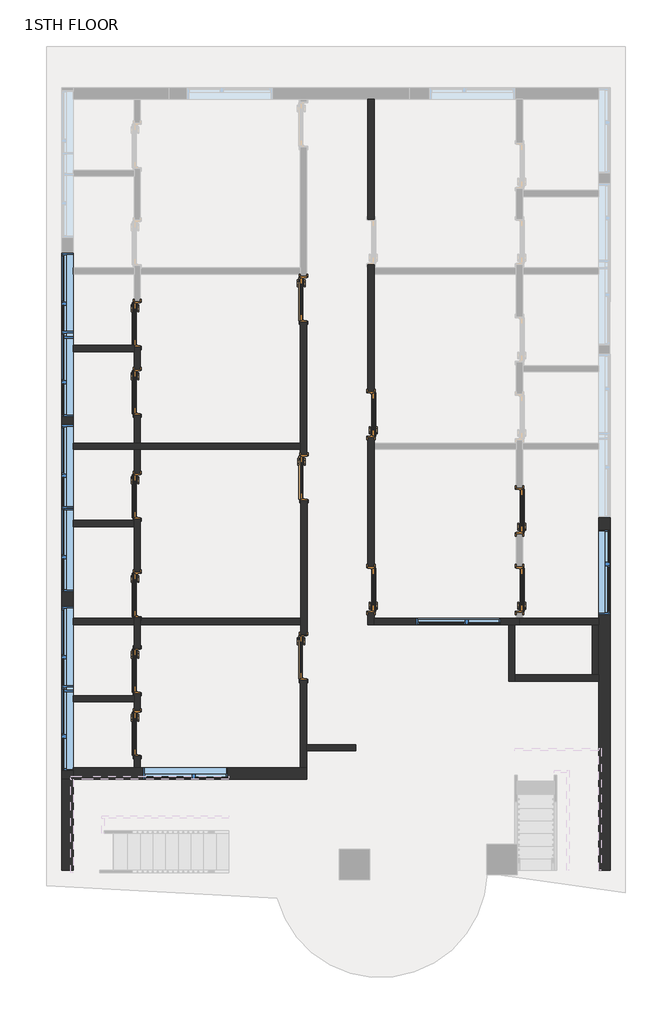
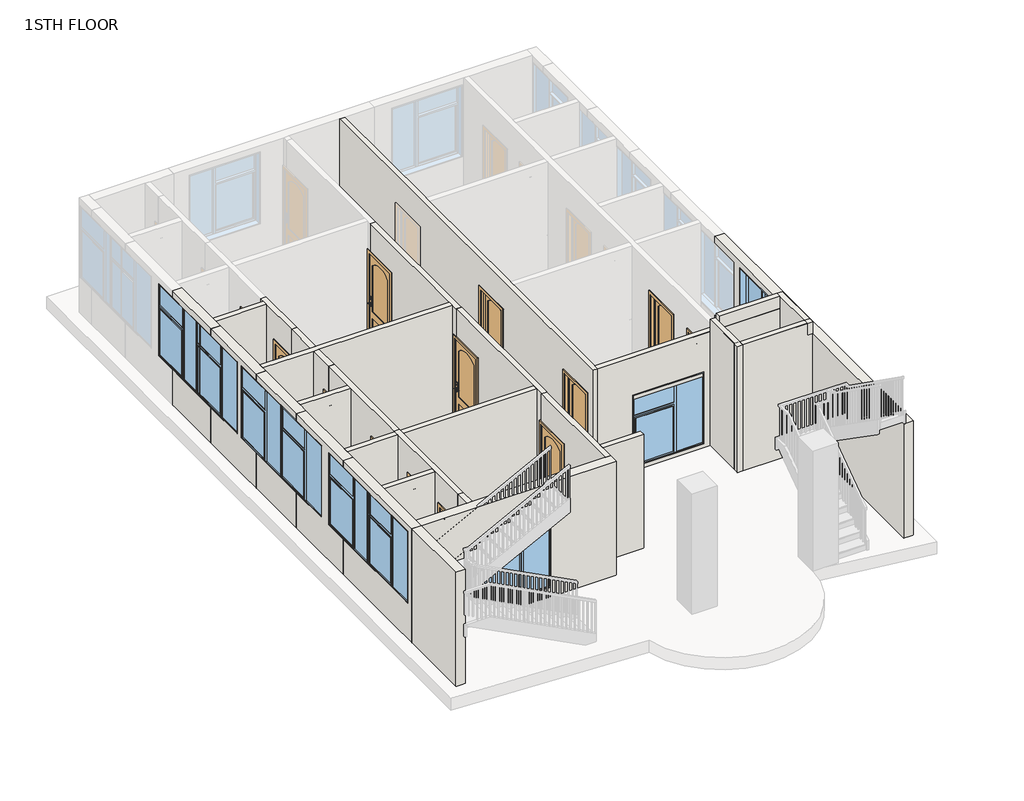
# One storey, part 1 of 4: 32 walls, 13 doors, 9 windows.
"""IFC4 building model written with IfcOpenShell, lengths in millimetres."""

from ifc_helpers import new_model, si_unit, frame, origin, place, context, project, spatial, polyline, outline, extrude, faceted_brep, transform, mapped, element, save
from components import door_346b4a94, m_window_casement_double_sidelight_1702_x_1829mm_c8b42c7f, m_window_casement_double_sidelight_1702_x_1829mm_92594323

model = new_model("IFC4")

# Units and contexts
model_context = context("Model", 3, world=origin())
ifc_project = project(units=[si_unit("LENGTHUNIT", "METRE", prefix="MILLI")], contexts=[model_context])

# Site, building, storey
site = spatial("IfcSite", under=ifc_project)
building = spatial("IfcBuilding", under=site)
storey = spatial("IfcBuildingStorey", under=building, Name="1STH FLOOR", Elevation=3200.4)

# Doors
placement = place(None, origin())
door_shape = door_346b4a94(model_context)
element("IfcDoor", 1, ObjectType="2'10\"X7'", at=placement, inside=storey, context=model_context, shape_type="MappedRepresentation", body=[
    mapped(door_shape, transform((2698.7641134, -459.3600272, 3200.4), x_axis=(0.0, -1.0, 0.0), y_axis=(1.0, 0.0, 0.0), z_axis=(0.0, 0.0, 1.0))),
])
element("IfcDoor", 2, ObjectType="2'10\"X7'", at=placement, inside=storey, context=model_context, shape_type="MappedRepresentation", body=[
    mapped(door_shape, transform((2698.7641134, -2034.1600272, 3200.4), x_axis=(0.0, -1.0, 0.0), y_axis=(1.0, 0.0, 0.0), z_axis=(0.0, 0.0, 1.0))),
])
element("IfcDoor", 3, ObjectType="2'10\"X7'", at=placement, inside=storey, context=model_context, shape_type="MappedRepresentation", body=[
    mapped(door_shape, transform((-273.0358866, -2034.1600272, 3200.4), x_axis=(0.0, -1.0, 0.0), y_axis=(1.0, 0.0, 0.0), z_axis=(0.0, 0.0, 1.0))),
])
element("IfcDoor", 4, ObjectType="2'10\"X7'", at=placement, inside=storey, context=model_context, shape_type="MappedRepresentation", body=[
    mapped(door_shape, transform((-273.0358866, 1471.0399728, 3200.4), x_axis=(0.0, -1.0, 0.0), y_axis=(1.0, 0.0, 0.0), z_axis=(0.0, 0.0, 1.0))),
])
element("IfcDoor", 5, ObjectType="2'10\"X7'", at=placement, inside=storey, context=model_context, shape_type="MappedRepresentation", body=[
    mapped(door_shape, transform((-4952.9858866, -3659.7600272, 3200.4), x_axis=(0.0, 1.0, 0.0), y_axis=(-1.0, 0.0, 0.0), z_axis=(0.0, 0.0, 1.0))),
])
element("IfcDoor", 6, ObjectType="2'10\"X7'", at=placement, inside=storey, context=model_context, shape_type="MappedRepresentation", body=[
    mapped(door_shape, transform((-4952.9858866, -2142.5151651, 3200.4), x_axis=(0.0, 1.0, 0.0), y_axis=(-1.0, 0.0, 0.0), z_axis=(0.0, 0.0, 1.0))),
])
element("IfcDoor", 7, ObjectType="2'10\"X7'", at=placement, inside=storey, context=model_context, shape_type="MappedRepresentation", body=[
    mapped(door_shape, transform((-4952.9858866, -167.9704957, 3200.4), x_axis=(0.0, 1.0, 0.0), y_axis=(-1.0, 0.0, 0.0), z_axis=(0.0, 0.0, 1.0))),
])
element("IfcDoor", 8, ObjectType="2'10\"X7'", at=placement, inside=storey, context=model_context, shape_type="MappedRepresentation", body=[
    mapped(door_shape, transform((-4952.9858866, 3273.6174518, 3200.4), x_axis=(0.0, 1.0, 0.0), y_axis=(-1.0, 0.0, 0.0), z_axis=(0.0, 0.0, 1.0))),
])
element("IfcDoor", 9, ObjectType="2'10\"X7'", at=placement, inside=storey, context=model_context, shape_type="MappedRepresentation", body=[
    mapped(door_shape, transform((-1625.1621817, 3775.8008884, 3200.4), x_axis=(0.0, 1.0, 0.0), y_axis=(-1.0, 0.0, 0.0), z_axis=(0.0, 0.0, 1.0))),
])
element("IfcDoor", 10, ObjectType="2'10\"X7'", at=placement, inside=storey, context=model_context, shape_type="MappedRepresentation", body=[
    mapped(door_shape, transform((-1629.1419858, -3390.4626067, 3200.4), x_axis=(0.0, 1.0, 0.0), y_axis=(-1.0, 0.0, 0.0), z_axis=(0.0, 0.0, 1.0))),
])
element("IfcDoor", 11, ObjectType="2'10\"X7'", at=placement, inside=storey, context=model_context, shape_type="MappedRepresentation", body=[
    mapped(door_shape, transform((-1620.1577262, 202.9637706, 3200.4), x_axis=(0.0, 1.0, 0.0), y_axis=(-1.0, 0.0, 0.0), z_axis=(0.0, 0.0, 1.0))),
])
element("IfcDoor", 12, ObjectType="2'10\"X7'", at=placement, inside=storey, context=model_context, shape_type="MappedRepresentation", body=[
    mapped(door_shape, transform((-4952.9858866, -4917.0600272, 3200.4), x_axis=(0.0, 1.0, 0.0), y_axis=(-1.0, 0.0, 0.0), z_axis=(0.0, 0.0, 1.0))),
])
element("IfcDoor", 13, ObjectType="2'10\"X7'", at=placement, inside=storey, context=model_context, shape_type="MappedRepresentation", body=[
    mapped(door_shape, transform((-4952.9858866, 1913.3521609, 3200.4), x_axis=(0.0, 1.0, 0.0), y_axis=(-1.0, 0.0, 0.0), z_axis=(0.0, 0.0, 1.0))),
])

# Walls
element("IfcWall", 14, ObjectType="Generic - 4.5\"", at=placement, inside=storey, context=model_context, shape_type="Brep", body=[
    faceted_brep([(-6232.5508078, 2728.3399728, 3200.4), (-5013.3108866, 2728.3399728, 3200.4), (-5013.3108866, 2728.3399728, 6096.0), (-6232.5508078, 2728.3399728, 6096.0), (-6232.5508078, 2855.3399728, 3200.4), (-6232.5508078, 2855.3399728, 6096.0), (-5013.3108866, 2855.3399728, 6096.0), (-5013.3108866, 2855.3399728, 3200.4), (-5013.3108866, 2816.8174518, 3200.4)], [[[0, 1, 2, 3]], [[4, 5, 6, 7]], [[1, 0, 4, 7, 8]], [[0, 3, 5, 4]], [[2, 1, 8, 7, 6]], [[3, 2, 6, 5]]]),
])
element("IfcWall", 15, ObjectType="Generic - 4.5\"", at=placement, inside=storey, context=model_context, shape_type="Brep", body=[
    faceted_brep([(-5013.3108866, 2968.8174518, 6096.0), (-5013.3108866, 2968.8174518, 5359.0), (-5013.3108866, 2816.8174518, 5359.0), (-5013.3108866, 2816.8174518, 3200.4), (-5013.3108866, 2728.3399728, 3200.4), (-5013.3108866, 2370.1521609, 3200.4), (-5013.3108866, 2370.1521609, 5359.0), (-5013.3108866, 1684.7521609, 5359.0), (-5013.3108866, 1684.7521609, 6096.0), (-5013.3108866, 2728.3399728, 6096.0), (-5013.3108866, 2855.3399728, 6096.0), (-4886.3108866, 2968.8174518, 5359.0), (-4886.3108866, 2968.8174518, 6096.0), (-4886.3108866, 1684.7521609, 6096.0), (-4886.3108866, 1684.7521609, 5359.0), (-4886.3108866, 2370.1521609, 5359.0), (-4886.3108866, 2370.1521609, 3200.4), (-4886.3108866, 2816.8174518, 3200.4), (-4886.3108866, 2816.8174518, 5359.0)], [[[0, 1, 2, 3, 4, 5, 6, 7, 8, 9, 10]], [[11, 12, 13, 14, 15, 16, 17, 18]], [[3, 17, 16, 5, 4]], [[13, 8, 7, 14]], [[1, 0, 12, 11]], [[18, 2, 1, 11]], [[2, 18, 17, 3]], [[15, 6, 5, 16]], [[6, 15, 14, 7]], [[0, 10, 9, 8, 13, 12]]]),
])
element("IfcWall", 16, ObjectType="Generic - 4.5\"", at=placement, inside=storey, context=model_context, shape_type="Brep", body=[
    faceted_brep([(-6232.5508078, 772.5399728, 3200.4), (-5013.3108866, 772.5399728, 3200.4), (-4886.3108866, 772.5399728, 3200.4), (-1685.9108866, 772.5399728, 3200.4), (-1685.9108866, 772.5399728, 6096.0), (-4886.3108866, 772.5399728, 6096.0), (-5013.3108866, 772.5399728, 6096.0), (-6232.5508078, 772.5399728, 6096.0), (-6232.5508078, 899.5399728, 3200.4), (-6232.5508078, 899.5399728, 6096.0), (-5013.3108866, 899.5399728, 6096.0), (-4886.3108866, 899.5399728, 6096.0), (-1685.9108866, 899.5399728, 6096.0), (-1685.9108866, 899.5399728, 3200.4), (-4886.3108866, 899.5399728, 3200.4), (-5013.3108866, 899.5399728, 3200.4)], [[[0, 1, 2, 3, 4, 5, 6, 7]], [[8, 9, 10, 11, 12, 13, 14, 15]], [[3, 2, 1, 0, 8, 15, 14, 13]], [[4, 3, 13, 12]], [[0, 7, 9, 8]], [[7, 6, 5, 4, 12, 11, 10, 9]]]),
])
element("IfcWall", 17, ObjectType="Generic - 4.5\"", at=placement, inside=storey, context=model_context, shape_type="SweptSolid", body=[
    extrude(outline(polyline([(136.8295043, 5359.0), (136.8295043, 6096.0), (772.5399728, 6096.0), (772.5399728, 3200.4), (288.8295043, 3200.4), (288.8295043, 5359.0), (136.8295043, 5359.0)])), frame((-5013.3108866, 0.0, 0.0), z_axis=(1.0, 0.0, 0.0), x_axis=(0.0, 1.0, 0.0)), (0.0, 0.0, 1.0), 127.0),
    extrude(outline(polyline([(1684.7521609, 6096.0), (1684.7521609, 5359.0), (1456.5521609, 5359.0), (1456.5521609, 3200.4), (899.5399728, 3200.4), (899.5399728, 6096.0), (1684.7521609, 6096.0)])), frame((-5013.3108866, 0.0, 0.0), z_axis=(1.0, 0.0, 0.0), x_axis=(0.0, 1.0, 0.0)), (0.0, 0.0, 1.0), 127.0),
])
element("IfcWall", 18, ObjectType="Generic - 4.5\"", at=placement, inside=storey, context=model_context, shape_type="SweptSolid", body=[
    extrude(outline(polyline([(-5013.3108866, -776.8600272), (-6232.5508078, -776.8600272), (-6232.5508078, -649.8600272), (-5013.3108866, -649.8600272), (-5013.3108866, -776.8600272)])), frame((0.0, 0.0, 3200.4), z_axis=(0.0, 0.0, 1.0), x_axis=(1.0, 0.0, 0.0)), (0.0, 0.0, 1.0), 2895.6),
])
element("IfcWall", 19, ObjectType="Generic - 4.5\"", at=placement, inside=storey, context=model_context, shape_type="Brep", body=[
    faceted_brep([(-5013.3108866, -2574.3151651, 5359.0), (-5013.3108866, -2574.3151651, 6096.0), (-5013.3108866, -776.8600272, 6096.0), (-5013.3108866, -649.8600272, 6096.0), (-5013.3108866, 136.8295043, 6096.0), (-5013.3108866, 136.8295043, 5359.0), (-5013.3108866, -624.7704957, 5359.0), (-5013.3108866, -624.7704957, 3200.4), (-5013.3108866, -649.8600272, 3200.4), (-5013.3108866, -776.8600272, 3200.4), (-5013.3108866, -1685.7151651, 3200.4), (-5013.3108866, -1685.7151651, 5359.0), (-4886.3108866, -2574.3151651, 6096.0), (-4886.3108866, -2574.3151651, 5359.0), (-4886.3108866, -1685.7151651, 5359.0), (-4886.3108866, -1685.7151651, 3200.4), (-4886.3108866, -624.7704957, 3200.4), (-4886.3108866, -624.7704957, 5359.0), (-4886.3108866, 136.8295043, 5359.0), (-4886.3108866, 136.8295043, 6096.0)], [[[0, 1, 2, 3, 4, 5, 6, 7, 8, 9, 10, 11]], [[12, 13, 14, 15, 16, 17, 18, 19]], [[15, 10, 9, 8, 7, 16]], [[1, 0, 13, 12]], [[4, 19, 18, 5]], [[14, 11, 10, 15]], [[11, 14, 13, 0]], [[17, 6, 5, 18]], [[6, 17, 16, 7]], [[4, 3, 2, 1, 12, 19]]]),
])
element("IfcWall", 20, ObjectType="Generic - 4.5\"", at=placement, inside=storey, context=model_context, shape_type="SweptSolid", body=[
    extrude(outline(polyline([(-5013.3108866, -2732.6600272), (-6232.5508078, -2732.6600272), (-6232.5508078, -2605.6600272), (-5013.3108866, -2605.6600272), (-5013.3108866, -2732.6600272)])), frame((0.0, 0.0, 3200.4), z_axis=(0.0, 0.0, 1.0), x_axis=(1.0, 0.0, 0.0)), (0.0, 0.0, 1.0), 2895.6),
])
element("IfcWall", 21, ObjectType="Generic - 4.5\"", at=placement, inside=storey, context=model_context, shape_type="Brep", body=[
    faceted_brep([(-5013.3108866, -3202.9600272, 3200.4), (-5013.3108866, -3202.9600272, 5359.0), (-5013.3108866, -4116.5600272, 5359.0), (-5013.3108866, -4116.5600272, 3200.4), (-5013.3108866, -4155.0600272, 3200.4), (-5013.3108866, -4282.0600272, 3200.4), (-5013.3108866, -4460.2600272, 3200.4), (-5013.3108866, -4460.2600272, 5359.0), (-5013.3108866, -5221.8600272, 5359.0), (-5013.3108866, -5221.8600272, 6096.0), (-5013.3108866, -4282.0600272, 6096.0), (-5013.3108866, -4155.0600272, 6096.0), (-5013.3108866, -2732.6600272, 6096.0), (-5013.3108866, -2605.6600272, 6096.0), (-5013.3108866, -2574.3151651, 6096.0), (-5013.3108866, -2574.3151651, 5359.0), (-5013.3108866, -2599.3151651, 5359.0), (-5013.3108866, -2599.3151651, 3200.4), (-5013.3108866, -2605.6600272, 3200.4), (-5013.3108866, -2732.6600272, 3200.4), (-4886.3108866, -3202.9600272, 5359.0), (-4886.3108866, -3202.9600272, 3200.4), (-4886.3108866, -2732.6600272, 3200.4), (-4886.3108866, -2605.6600272, 3200.4), (-4886.3108866, -2599.3151651, 3200.4), (-4886.3108866, -2599.3151651, 5359.0), (-4886.3108866, -2574.3151651, 5359.0), (-4886.3108866, -2574.3151651, 6096.0), (-4886.3108866, -2605.6600272, 6096.0), (-4886.3108866, -2732.6600272, 6096.0), (-4886.3108866, -5221.8600272, 6096.0), (-4886.3108866, -5221.8600272, 5359.0), (-4886.3108866, -4460.2600272, 5359.0), (-4886.3108866, -4460.2600272, 3200.4), (-4886.3108866, -4116.5600272, 3200.4), (-4886.3108866, -4116.5600272, 5359.0)], [[[0, 1, 2, 3, 4, 5, 6, 7, 8, 9, 10, 11, 12, 13, 14, 15, 16, 17, 18, 19]], [[20, 21, 22, 23, 24, 25, 26, 27, 28, 29, 30, 31, 32, 33, 34, 35]], [[21, 0, 19, 18, 17, 24, 23, 22]], [[3, 34, 33, 6, 5, 4]], [[30, 9, 8, 31]], [[15, 14, 27, 26]], [[20, 1, 0, 21]], [[1, 20, 35, 2]], [[2, 35, 34, 3]], [[25, 16, 15, 26]], [[16, 25, 24, 17]], [[32, 7, 6, 33]], [[7, 32, 31, 8]], [[14, 13, 12, 11, 10, 9, 30, 29, 28, 27]]]),
])
element("IfcWall", 22, ObjectType="Generic - 4.5\"", at=placement, inside=storey, context=model_context, shape_type="SweptSolid", body=[
    extrude(outline(polyline([(-5013.3108866, -4282.0600272), (-6232.5324766, -4282.0600272), (-6232.5342541, -4155.0600272), (-5013.3108866, -4155.0600272), (-5013.3108866, -4282.0600272)])), frame((0.0, 0.0, 3200.4), z_axis=(0.0, 0.0, 1.0), x_axis=(1.0, 0.0, 0.0)), (0.0, 0.0, 1.0), 2895.6),
])
element("IfcWall", 23, ObjectType="Generic - 4.5\"", at=placement, inside=storey, context=model_context, shape_type="SweptSolid", body=[
    extrude(outline(polyline([(-1685.9108866, -2732.6600272), (-4886.3108866, -2732.6600272), (-4886.3108866, -2605.6600272), (-1685.9108866, -2605.6600272), (-1685.9108866, -2732.6600272)])), frame((0.0, 0.0, 3200.4), z_axis=(0.0, 0.0, 1.0), x_axis=(1.0, 0.0, 0.0)), (0.0, 0.0, 1.0), 2895.6),
])
element("IfcWall", 24, ObjectType="Generic - 4.5\"", at=placement, inside=storey, context=model_context, shape_type="Brep", body=[
    faceted_brep([(-1685.4871817, 4182.2008884, 6096.0), (-1685.4871817, 4182.2008884, 5359.0), (-1685.4871817, 3319.0008884, 5359.0), (-1685.4871817, 3319.0008884, 3200.4), (-1685.4871817, 659.7637706, 3200.4), (-1685.4871817, 659.7637706, 5359.0), (-1685.4871817, 609.3637706, 5359.0), (-1685.4871817, 609.3637706, 6096.0), (-1558.4871817, 4182.2008884, 5359.0), (-1558.4871817, 4182.2008884, 6096.0), (-1558.4871817, 609.3637706, 6096.0), (-1558.4871817, 609.3637706, 5359.0), (-1558.4871817, 659.7637706, 5359.0), (-1558.4871817, 659.7637706, 3200.4), (-1558.4871817, 3319.0008884, 3200.4), (-1558.4871817, 3319.0008884, 5359.0), (-1680.4827262, 609.3637706, 6096.0), (-1680.4827262, 609.3637706, 5359.0), (-1558.9108866, 4182.2008884, 6096.0), (-1558.9108866, 4182.2008884, 5359.0)], [[[0, 1, 2, 3, 4, 5, 6, 7]], [[8, 9, 10, 11, 12, 13, 14, 15]], [[3, 14, 13, 4]], [[10, 16, 7, 6, 17, 11]], [[1, 0, 18, 9, 8, 19]], [[15, 2, 1, 19, 8]], [[2, 15, 14, 3]], [[12, 5, 4, 13]], [[5, 12, 11, 17, 6]], [[0, 7, 16, 10, 9, 18]]]),
])
element("IfcWall", 25, ObjectType="Generic - 4.5\"", at=placement, inside=storey, context=model_context, shape_type="Brep", body=[
    faceted_brep([(-1680.4827262, -2933.2626067, 3200.4), (-1680.4827262, -2933.2626067, 6096.0), (-1680.4827262, 609.3637706, 6096.0), (-1680.4827262, 609.3637706, 5359.0), (-1680.4827262, -253.8362294, 5359.0), (-1680.4827262, -253.8362294, 3200.4), (-1553.4827262, -2933.2626067, 6096.0), (-1553.4827262, -2933.2626067, 3200.4), (-1553.4827262, -253.8362294, 3200.4), (-1553.4827262, -253.8362294, 5359.0), (-1553.4827262, 609.3637706, 5359.0), (-1553.4827262, 609.3637706, 6096.0), (-1562.4669858, -2933.2626067, 3200.4), (-1562.4669858, -2933.2626067, 6096.0), (-1558.4871817, 609.3637706, 6096.0), (-1558.4871817, 609.3637706, 5359.0)], [[[0, 1, 2, 3, 4, 5]], [[6, 7, 8, 9, 10, 11]], [[7, 12, 0, 5, 8]], [[1, 0, 12, 7, 6, 13]], [[2, 14, 11, 10, 15, 3]], [[9, 4, 3, 15, 10]], [[4, 9, 8, 5]], [[2, 1, 13, 6, 11, 14]]]),
])
element("IfcWall", 26, ObjectType="Generic - 4.5\"", at=placement, inside=storey, context=model_context, shape_type="Brep", body=[
    faceted_brep([(-1689.4669858, -2933.2626067, 6096.0), (-1689.4669858, -2933.2626067, 3200.4), (-1689.4669858, -2933.6626067, 3200.4), (-1689.4669858, -2933.6626067, 5359.0), (-1689.4669858, -3847.2626067, 5359.0), (-1689.4669858, -3847.2626067, 3200.4), (-1689.4669858, -5596.1082131, 3200.4), (-1689.4669858, -5596.1082131, 6096.0), (-1562.4669858, -2933.2626067, 3200.4), (-1562.4669858, -2933.2626067, 6096.0), (-1562.4669858, -5136.3822004, 6096.0), (-1562.4669858, -5263.3822004, 6096.0), (-1562.4669858, -5596.1082131, 6096.0), (-1562.4669858, -5596.1082131, 3200.4), (-1562.4669858, -5263.3822004, 3200.4), (-1562.4669858, -5136.3822004, 3200.4), (-1562.4669858, -3847.2626067, 3200.4), (-1562.4669858, -3847.2626067, 5359.0), (-1562.4669858, -2933.6626067, 5359.0), (-1562.4669858, -2933.6626067, 3200.4), (-1680.4827262, -2933.2626067, 3200.4), (-1680.4827262, -2933.2626067, 6096.0)], [[[0, 1, 2, 3, 4, 5, 6, 7]], [[8, 9, 10, 11, 12, 13, 14, 15, 16, 17, 18, 19]], [[1, 20, 8, 19, 2]], [[13, 6, 5, 16, 15, 14]], [[1, 0, 21, 9, 8, 20]], [[18, 3, 2, 19]], [[3, 18, 17, 4]], [[4, 17, 16, 5]], [[7, 6, 13, 12]], [[0, 7, 12, 11, 10, 9, 21]]]),
])
element("IfcWall", 27, ObjectType="Generic - 4.5\"", at=placement, inside=storey, context=model_context, shape_type="Brep", body=[
    faceted_brep([(-339.7108866, 7782.9399728, 6096.0), (-339.7108866, 7782.9399728, 3200.4), (-339.7108866, 5382.2399728, 3200.4), (-339.7108866, 5382.2399728, 5359.0), (-339.7108866, 4468.6399728, 5359.0), (-339.7108866, 4468.6399728, 3200.4), (-339.7108866, 1927.8399728, 3200.4), (-339.7108866, 1927.8399728, 5359.0), (-339.7108866, 1014.2399728, 5359.0), (-339.7108866, 1014.2399728, 3200.4), (-339.7108866, -1577.3600272, 3200.4), (-339.7108866, -1577.3600272, 5359.0), (-339.7108866, -2490.9600272, 5359.0), (-339.7108866, -2490.9600272, 3200.4), (-339.7108866, -2732.6600272, 3200.4), (-339.7108866, -2732.6600272, 6096.0), (-212.7108866, 7782.9399728, 3200.4), (-212.7108866, 7782.9399728, 6096.0), (-212.7108866, 4404.7399728, 6096.0), (-212.7108866, 4277.7399728, 6096.0), (-212.7108866, 899.5399728, 6096.0), (-212.7108866, 772.5399728, 6096.0), (-212.7108866, -2605.6600272, 6096.0), (-212.7108866, -2732.6600272, 6096.0), (-212.7108866, -2732.6600272, 3200.4), (-212.7108866, -2605.6600272, 3200.4), (-212.7108866, -2490.9600272, 3200.4), (-212.7108866, -2490.9600272, 5359.0), (-212.7108866, -1577.3600272, 5359.0), (-212.7108866, -1577.3600272, 3200.4), (-212.7108866, 772.5399728, 3200.4), (-212.7108866, 899.5399728, 3200.4), (-212.7108866, 1014.2399728, 3200.4), (-212.7108866, 1014.2399728, 5359.0), (-212.7108866, 1927.8399728, 5359.0), (-212.7108866, 1927.8399728, 3200.4), (-212.7108866, 4277.7399728, 3200.4), (-212.7108866, 4404.7399728, 3200.4), (-212.7108866, 4468.6399728, 3200.4), (-212.7108866, 4468.6399728, 5359.0), (-212.7108866, 5382.2399728, 5359.0), (-212.7108866, 5382.2399728, 3200.4)], [[[0, 1, 2, 3, 4, 5, 6, 7, 8, 9, 10, 11, 12, 13, 14, 15]], [[16, 17, 18, 19, 20, 21, 22, 23, 24, 25, 26, 27, 28, 29, 30, 31, 32, 33, 34, 35, 36, 37, 38, 39, 40, 41]], [[1, 16, 41, 2]], [[24, 14, 13, 26, 25]], [[29, 10, 9, 32, 31, 30]], [[35, 6, 5, 38, 37, 36]], [[1, 0, 17, 16]], [[15, 14, 24, 23]], [[12, 27, 26, 13]], [[27, 12, 11, 28]], [[28, 11, 10, 29]], [[8, 33, 32, 9]], [[33, 8, 7, 34]], [[34, 7, 6, 35]], [[4, 39, 38, 5]], [[39, 4, 3, 40]], [[40, 3, 2, 41]], [[0, 15, 23, 22, 21, 20, 19, 18, 17]]]),
])
element("IfcWall", 28, ObjectType="Generic - 4.5\"", at=placement, inside=storey, context=model_context, shape_type="Brep", body=[
    faceted_brep([(-212.7108866, -2732.6600272, 6096.0), (-212.7108866, -2732.6600272, 3200.4), (625.4891134, -2732.6600272, 3200.4), (625.4891134, -2732.6600272, 5014.5114654), (2327.2891134, -2732.6600272, 5014.5114654), (2327.2891134, -2732.6600272, 3200.4), (2479.6891134, -2732.6600272, 3200.4), (2606.6891134, -2732.6600272, 3200.4), (4281.7311655, -2732.6600272, 3200.4), (4281.7311655, -2732.6600272, 6096.0), (-212.7108866, -2605.6600272, 3200.4), (-212.7108866, -2605.6600272, 6096.0), (2632.0891134, -2605.6600272, 6096.0), (2759.0891134, -2605.6600272, 6096.0), (4281.7311655, -2605.6600272, 6096.0), (4281.7311655, -2605.6600272, 3200.4), (2759.0891134, -2605.6600272, 3200.4), (2632.0891134, -2605.6600272, 3200.4), (2327.2891134, -2605.6600272, 3200.4), (2327.2891134, -2605.6600272, 5014.5114654), (625.4891134, -2605.6600272, 5014.5114654), (625.4891134, -2605.6600272, 3200.4)], [[[0, 1, 2, 3, 4, 5, 6, 7, 8, 9]], [[10, 11, 12, 13, 14, 15, 16, 17, 18, 19, 20, 21]], [[1, 10, 21, 2]], [[15, 8, 7, 6, 5, 18, 17, 16]], [[1, 0, 11, 10]], [[9, 8, 15, 14]], [[0, 9, 14, 13, 12, 11]], [[20, 3, 2, 21]], [[4, 19, 18, 5]], [[3, 20, 19, 4]]]),
])
element("IfcWall", 29, ObjectType="Generic - 4.5\"", at=placement, inside=storey, context=model_context, shape_type="Brep", body=[
    faceted_brep([(-212.7108866, -2732.6600272, 3200.4), (2479.6891134, -2732.6600272, 3200.4), (2606.6891134, -2732.6600272, 3200.4), (2695.5891134, -2732.6600272, 3200.4), (2695.5891134, -2732.6600272, 6096.0), (-212.7108866, -2732.6600272, 6096.0), (625.4891134, -2732.6600272, 5126.3883506), (2327.2891134, -2732.6600272, 5126.3883506), (2327.2891134, -2732.6600272, 3297.5883506), (625.4891134, -2732.6600272, 3297.5883506), (-212.7108866, -2605.6600272, 3200.4), (-212.7108866, -2605.6600272, 6096.0), (2632.0891134, -2605.6600272, 6096.0), (2695.5891134, -2605.6600272, 6096.0), (2695.5891134, -2605.6600272, 3200.4), (2632.0891134, -2605.6600272, 3200.4), (625.4891134, -2605.6600272, 5126.3883506), (625.4891134, -2605.6600272, 3297.5883506), (2327.2891134, -2605.6600272, 3297.5883506), (2327.2891134, -2605.6600272, 5126.3883506)], [[[0, 1, 2, 3, 4, 5], [6, 7, 8, 9]], [[10, 11, 12, 13, 14, 15], [16, 17, 18, 19]], [[3, 2, 1, 0, 10, 15, 14]], [[4, 3, 14, 13]], [[5, 4, 13, 12, 11]], [[17, 16, 6, 9]], [[18, 17, 9, 8]], [[19, 18, 8, 7]], [[16, 19, 7, 6]], [[0, 5, 11, 10]]]),
])
element("IfcWall", 30, ObjectType="Generic - 5\"", at=placement, inside=storey, context=model_context, shape_type="SweptSolid", body=[
    extrude(outline(polyline([(-5593.5822004, 3200.4), (-5593.5822004, 6096.0), (-5221.8600272, 6096.0), (-5221.8600272, 5359.0), (-5373.8600272, 5359.0), (-5373.8600272, 3200.4), (-5593.5822004, 3200.4)])), frame((-5013.3108866, 0.0, 0.0), z_axis=(1.0, 0.0, 0.0), x_axis=(0.0, 1.0, 0.0)), (0.0, 0.0, 1.0), 127.0),
])
element("IfcWall", 31, ObjectType="Generic - 5\"", at=placement, inside=storey, context=model_context, shape_type="SweptSolid", body=[
    extrude(outline(polyline([(-1562.4669858, -5136.3822004), (-581.0108866, -5136.3822004), (-581.0108866, -5263.3822004), (-1562.4669858, -5263.3822004), (-1562.4669858, -5136.3822004)])), frame((0.0, 0.0, 3200.4), z_axis=(0.0, 0.0, 1.0), x_axis=(1.0, 0.0, 0.0)), (0.0, 0.0, 1.0), 2895.6),
])
element("IfcWall", 32, ObjectType="Generic - 5\"", at=placement, inside=storey, context=model_context, shape_type="Brep", body=[
    faceted_brep([(2479.6891134, -2732.6600272, 3200.4), (2479.6891134, -3866.3822004, 3200.4), (2479.6891134, -3866.3822004, 6400.8), (2479.6891134, -2732.6600272, 6400.8), (2606.6891134, -2732.6600272, 3200.4), (2606.6891134, -2732.6600272, 6400.8), (2606.6891134, -3739.3822004, 6400.8), (2606.6891134, -3866.3822004, 6400.8), (2606.6891134, -3866.3822004, 3200.4), (2606.6891134, -3739.3822004, 3200.4)], [[[0, 1, 2, 3]], [[4, 5, 6, 7, 8, 9]], [[1, 0, 4, 9, 8]], [[3, 2, 7, 6, 5]], [[2, 1, 8, 7]], [[0, 3, 5, 4]]]),
])
element("IfcWall", 33, ObjectType="Generic - 5\"", at=placement, inside=storey, context=model_context, shape_type="Brep", body=[
    faceted_brep([(2606.6891134, -3866.3822004, 3200.4), (4281.7311655, -3866.3822004, 3200.4), (4281.7311655, -3866.3822004, 6096.0), (4154.7311655, -3866.3822004, 6096.0), (4154.7311655, -3866.3822004, 6400.8), (2606.6891134, -3866.3822004, 6400.8), (2606.6891134, -3739.3822004, 3200.4), (2606.6891134, -3739.3822004, 6400.8), (4154.7311655, -3739.3822004, 6400.8), (4154.7311655, -3739.3822004, 6096.0), (4281.7311655, -3739.3822004, 6096.0), (4281.7311655, -3739.3822004, 3200.4), (4154.7311655, -3739.3822004, 3200.4)], [[[0, 1, 2, 3, 4, 5]], [[6, 7, 8, 9, 10, 11, 12]], [[1, 0, 6, 12, 11]], [[5, 4, 8, 7]], [[0, 5, 7, 6]], [[9, 3, 2, 10]], [[2, 1, 11, 10]], [[4, 3, 9, 8]]]),
])
element("IfcWall", 34, ObjectType="Generic - 5\"", at=placement, inside=storey, context=model_context, shape_type="SweptSolid", body=[
    extrude(outline(polyline([(2479.6891134, -3739.3822004), (2479.6891134, -2732.6600272), (2606.6891134, -2732.6600272), (2606.6891134, -3739.3822004), (2479.6891134, -3739.3822004)])), frame((0.0, 0.0, 3200.4), z_axis=(0.0, 0.0, 1.0), x_axis=(1.0, 0.0, 0.0)), (0.0, 0.0, 1.0), 3200.4),
])
element("IfcWall", 35, ObjectType="Generic - 5\"", at=placement, inside=storey, context=model_context, shape_type="Brep", body=[
    faceted_brep([(2606.6891134, -3866.3822004, 3200.4), (4281.7311655, -3866.3822004, 3200.4), (4281.7311655, -3866.3822004, 6400.8), (2606.6891134, -3866.3822004, 6400.8), (2606.6891134, -3739.3822004, 3200.4), (2606.6891134, -3739.3822004, 6400.8), (4154.7311655, -3739.3822004, 6400.8), (4281.7311655, -3739.3822004, 6400.8), (4281.7311655, -3739.3822004, 3200.4), (4154.7311655, -3739.3822004, 3200.4)], [[[0, 1, 2, 3]], [[4, 5, 6, 7, 8, 9]], [[1, 0, 4, 9, 8]], [[3, 2, 7, 6, 5]], [[2, 1, 8, 7]], [[0, 3, 5, 4]]]),
])
element("IfcWall", 36, ObjectType="Generic - 5\"", at=placement, inside=storey, context=model_context, shape_type="Brep", body=[
    faceted_brep([(4281.7311655, -3739.3822004, 3200.4), (4281.7311655, -2605.6600272, 3200.4), (4281.7311655, -2605.6600272, 6400.8), (4281.7311655, -3739.3822004, 6400.8), (4281.7311655, -3739.3822004, 6096.0), (4154.7311655, -3739.3822004, 3200.4), (4154.7311655, -3739.3822004, 6400.8), (4154.7311655, -2732.6600272, 6400.8), (4154.7311655, -2605.6600272, 6400.8), (4154.7311655, -2605.6600272, 3200.4), (4154.7311655, -2732.6600272, 3200.4)], [[[0, 1, 2, 3, 4]], [[5, 6, 7, 8, 9, 10]], [[1, 0, 5, 10, 9]], [[3, 2, 8, 7, 6]], [[0, 4, 3, 6, 5]], [[1, 9, 8, 2]]]),
])
element("IfcWall", 37, ObjectType="Generic - 5\"", at=placement, inside=storey, context=model_context, shape_type="Brep", body=[
    faceted_brep([(2695.5891134, -2732.6600272, 3200.4), (4154.7311655, -2732.6600272, 3200.4), (4154.7311655, -2732.6600272, 6400.8), (2695.5891134, -2732.6600272, 6400.8), (2695.5891134, -2732.6600272, 6096.0), (2695.5891134, -2605.6600272, 3200.4), (2695.5891134, -2605.6600272, 6096.0), (2695.5891134, -2605.6600272, 6400.8), (4154.7311655, -2605.6600272, 6400.8), (4154.7311655, -2605.6600272, 3200.4), (2759.0891134, -2605.6600272, 3200.4)], [[[0, 1, 2, 3, 4]], [[5, 6, 7, 8, 9, 10]], [[1, 0, 5, 10, 9]], [[3, 2, 8, 7]], [[0, 4, 3, 7, 6, 5]], [[2, 1, 9, 8]]]),
])
element("IfcWall", 38, ObjectType="Generic - 9\"", at=placement, inside=storey, context=model_context, shape_type="Brep", body=[
    faceted_brep([(4281.7311655, 200.5184135, 3200.4), (4281.7311655, -2605.6600272, 3200.4), (4281.7311655, -2732.6600272, 3200.4), (4281.7311655, -3739.3822004, 3200.4), (4281.7311655, -3866.3822004, 3200.4), (4281.7311655, -7650.9822004, 3200.4), (4281.7311655, -7650.9822004, 6096.0), (4281.7311655, -3866.3822004, 6096.0), (4281.7311655, -3739.3822004, 6096.0), (4281.7311655, -2732.6600272, 6096.0), (4281.7311655, -2605.6600272, 6096.0), (4281.7311655, 200.5184135, 6096.0), (4281.7311655, 200.5184135, 5929.2), (4281.7311655, -599.0600272, 5929.2), (4281.7311655, -599.0600272, 4100.4), (4281.7311655, 200.5184135, 4100.4), (4281.7311655, -2537.537179, 4100.4), (4281.7311655, -835.737179, 4100.4), (4281.7311655, -835.737179, 5929.2), (4281.7311655, -2537.537179, 5929.2), (4510.3311655, -7650.9822004, 3200.4), (4510.3311655, 200.5184135, 3200.4), (4510.3311655, 200.5184135, 4100.4), (4510.3311655, -599.0600272, 4100.4), (4510.3311655, -599.0600272, 5929.2), (4510.3311655, 200.5184135, 5929.2), (4510.3311655, 200.5184135, 6096.0), (4510.3311655, -7650.9822004, 6096.0), (4510.3311655, -835.737179, 4100.4), (4510.3311655, -2537.537179, 4100.4), (4510.3311655, -2537.537179, 5929.2), (4510.3311655, -835.737179, 5929.2), (4283.0918814, 200.5184135, 3200.4), (4283.0918814, 200.5184135, 4100.4), (4283.0918814, 200.5184135, 6096.0), (4283.0918814, 200.5184135, 5929.2)], [[[0, 1, 2, 3, 4, 5, 6, 7, 8, 9, 10, 11, 12, 13, 14, 15], [16, 17, 18, 19]], [[20, 21, 22, 23, 24, 25, 26, 27], [28, 29, 30, 31]], [[5, 4, 3, 2, 1, 0, 32, 21, 20]], [[6, 5, 20, 27]], [[21, 32, 0, 15, 33, 22]], [[12, 11, 34, 26, 25, 35]], [[13, 24, 23, 14]], [[14, 23, 22, 33, 15]], [[24, 13, 12, 35, 25]], [[16, 29, 28, 17]], [[17, 28, 31, 18]], [[18, 31, 30, 19]], [[29, 16, 19, 30]], [[11, 10, 9, 8, 7, 6, 27, 26, 34]]]),
])
element("IfcWall", 39, ObjectType="Generic - 9\"", at=placement, inside=storey, context=model_context, shape_type="Brep", body=[
    faceted_brep([(-6232.5108866, -5824.7082131, 3200.4), (-6232.5140859, -5596.1082131, 3200.4), (-6232.5324766, -4282.0600272, 3200.4), (-6232.5342541, -4155.0600272, 3200.4), (-6232.5508078, -2972.263382, 3200.4), (-6232.5508078, -2972.263382, 4100.4), (-6232.5131972, -5659.6082132, 4100.4), (-6232.5131972, -5659.6082132, 5929.2), (-6232.5508078, -2972.263382, 5929.2), (-6232.5508078, -2972.263382, 6096.0), (-6232.5342541, -4155.0600272, 6096.0), (-6232.5324766, -4282.0600272, 6096.0), (-6232.5140859, -5596.1082131, 6096.0), (-6232.5108866, -5824.7082131, 6096.0), (-6461.1508078, -2972.2665814, 3200.4), (-6461.1108866, -5824.7082131, 3200.4), (-6461.1108866, -5824.7082131, 6096.0), (-6461.1508078, -2972.2665814, 6096.0), (-6461.1508078, -2972.2665814, 5929.2), (-6461.1131972, -5659.6114126, 5929.2), (-6461.1131972, -5659.6114126, 4100.4), (-6461.1508078, -2972.2665814, 4100.4)], [[[0, 1, 2, 3, 4, 5, 6, 7, 8, 9, 10, 11, 12, 13]], [[14, 15, 16, 17, 18, 19, 20, 21]], [[4, 3, 2, 1, 0, 15, 14]], [[4, 14, 21, 5]], [[9, 8, 18, 17]], [[5, 21, 20, 6]], [[18, 8, 7, 19]], [[19, 7, 6, 20]], [[0, 13, 16, 15]], [[13, 12, 11, 10, 9, 17, 16]]]),
])
element("IfcWall", 40, ObjectType="Generic - 9\"", at=placement, inside=storey, context=model_context, shape_type="Brep", body=[
    faceted_brep([(-6232.5508078, -2972.2649817, 3200.4), (-6232.5508078, -2732.6600272, 3200.4), (-6232.5508078, -2605.6600272, 3200.4), (-6232.5508078, -1019.7048138, 3200.4), (-6232.5508078, -1019.7048138, 4100.4), (-6232.5508078, -2073.8048138, 4100.4), (-6232.5508078, -2073.8048138, 5929.2), (-6232.5508078, -1019.7048138, 5929.2), (-6232.5508078, -1019.7048138, 6096.0), (-6232.5508078, -2605.6600272, 6096.0), (-6232.5508078, -2732.6600272, 6096.0), (-6232.5508078, -2972.2649817, 6096.0), (-6232.5508078, -2972.2649817, 5929.2), (-6232.5508078, -2375.3633819, 5929.2), (-6232.5508078, -2375.3633819, 4100.4), (-6232.5508078, -2972.2649817, 4100.4), (-6461.1508078, -1019.7048138, 3200.4), (-6461.1508078, -2972.2649817, 3200.4), (-6461.1508078, -2972.2649817, 4100.4), (-6461.1508078, -2375.3665813, 4100.4), (-6461.1508078, -2375.3665813, 5929.2), (-6461.1508078, -2972.2649817, 5929.2), (-6461.1508078, -2972.2649817, 6096.0), (-6461.1508078, -1019.7048138, 6096.0), (-6461.1508078, -1019.7048138, 5929.2), (-6461.1508078, -2073.8048138, 5929.2), (-6461.1508078, -2073.8048138, 4100.4), (-6461.1508078, -1019.7048138, 4100.4)], [[[0, 1, 2, 3, 4, 5, 6, 7, 8, 9, 10, 11, 12, 13, 14, 15]], [[16, 17, 18, 19, 20, 21, 22, 23, 24, 25, 26, 27]], [[3, 2, 1, 0, 17, 16]], [[3, 16, 27, 4]], [[8, 7, 24, 23]], [[17, 0, 15, 18]], [[11, 22, 21, 12]], [[26, 5, 4, 27]], [[5, 26, 25, 6]], [[6, 25, 24, 7]], [[13, 20, 19, 14]], [[14, 19, 18, 15]], [[20, 13, 12, 21]], [[11, 10, 9, 8, 23, 22]]]),
])
element("IfcWall", 41, ObjectType="Generic - 9\"", at=placement, inside=storey, context=model_context, shape_type="Brep", body=[
    faceted_brep([(-6232.5508078, -1019.7048138, 3200.4), (-6232.5508078, -776.8600272, 3200.4), (-6232.5508078, -649.8600272, 3200.4), (-6232.5508078, 642.0011338, 3200.4), (-6232.5508078, 642.0011338, 4100.4), (-6232.5508078, -1019.7048138, 4100.4), (-6461.1508078, 642.0011338, 3200.4), (-6461.1508078, -1019.7048138, 3200.4), (-6461.1508078, -1019.7048138, 4100.4), (-6461.1508078, 642.0011338, 4100.4)], [[[0, 1, 2, 3, 4, 5]], [[6, 7, 8, 9]], [[3, 2, 1, 0, 7, 6]], [[3, 6, 9, 4]], [[7, 0, 5, 8]], [[4, 9, 8, 5]]]),
    faceted_brep([(-6232.5508078, -1019.7048138, 5929.2), (-6232.5508078, 642.0011338, 5929.2), (-6232.5508078, 642.0011338, 6096.0), (-6232.5508078, -649.8600272, 6096.0), (-6232.5508078, -776.8600272, 6096.0), (-6232.5508078, -1019.7048138, 6096.0), (-6461.1508078, 642.0011338, 6096.0), (-6461.1508078, 642.0011338, 5929.2), (-6461.1508078, -1019.7048138, 5929.2), (-6461.1508078, -1019.7048138, 6096.0)], [[[0, 1, 2, 3, 4, 5]], [[6, 7, 8, 9]], [[2, 1, 7, 6]], [[5, 9, 8, 0]], [[7, 1, 0, 8]], [[5, 4, 3, 2, 6, 9]]]),
])
element("IfcWall", 42, ObjectType="Generic - 9\"", at=placement, inside=storey, context=model_context, shape_type="Brep", body=[
    faceted_brep([(-6232.5508078, 642.0011338, 3200.4), (-6232.5508078, 772.5399728, 3200.4), (-6232.5508078, 899.5399728, 3200.4), (-6232.5508078, 2534.5107865, 3200.4), (-6232.5508078, 2534.5107865, 4100.4), (-6232.5508078, 1429.6107865, 4100.4), (-6232.5508078, 1429.6107865, 5929.2), (-6232.5508078, 2534.5107865, 5929.2), (-6232.5508078, 2534.5107865, 6096.0), (-6232.5508078, 899.5399728, 6096.0), (-6232.5508078, 772.5399728, 6096.0), (-6232.5508078, 642.0011338, 6096.0), (-6232.5508078, 642.0011338, 5929.2), (-6232.5508078, 1264.3011338, 5929.2), (-6232.5508078, 1264.3011338, 4100.4), (-6232.5508078, 642.0011338, 4100.4), (-6461.1508078, 2534.5107865, 3200.4), (-6461.1508078, 642.0011338, 3200.4), (-6461.1508078, 642.0011338, 4100.4), (-6461.1508078, 1264.3011338, 4100.4), (-6461.1508078, 1264.3011338, 5929.2), (-6461.1508078, 642.0011338, 5929.2), (-6461.1508078, 642.0011338, 6096.0), (-6461.1508078, 2534.5107865, 6096.0), (-6461.1508078, 2534.5107865, 5929.2), (-6461.1508078, 1429.6107865, 5929.2), (-6461.1508078, 1429.6107865, 4100.4), (-6461.1508078, 2534.5107865, 4100.4)], [[[0, 1, 2, 3, 4, 5, 6, 7, 8, 9, 10, 11, 12, 13, 14, 15]], [[16, 17, 18, 19, 20, 21, 22, 23, 24, 25, 26, 27]], [[3, 2, 1, 0, 17, 16]], [[3, 16, 27, 4]], [[8, 7, 24, 23]], [[17, 0, 15, 18]], [[11, 22, 21, 12]], [[26, 5, 4, 27]], [[5, 26, 25, 6]], [[6, 25, 24, 7]], [[13, 20, 19, 14]], [[14, 19, 18, 15]], [[20, 13, 12, 21]], [[11, 10, 9, 8, 23, 22]]]),
])
element("IfcWall", 43, ObjectType="Generic - 9\"", at=placement, inside=storey, context=model_context, shape_type="Brep", body=[
    faceted_brep([(-6232.5508078, 2534.5107865, 3200.4), (-6232.5508078, 2728.3399728, 3200.4), (-6232.5508078, 2855.3399728, 3200.4), (-6232.5508078, 4130.2388609, 3200.4), (-6232.5508078, 4130.2388609, 4100.4), (-6232.5508078, 2534.5107865, 4100.4), (-6461.1508078, 4130.2388609, 3200.4), (-6461.1508078, 2534.5107865, 3200.4), (-6461.1508078, 2534.5107865, 4100.4), (-6461.1508078, 4130.2388609, 4100.4)], [[[0, 1, 2, 3, 4, 5]], [[6, 7, 8, 9]], [[3, 2, 1, 0, 7, 6]], [[3, 6, 9, 4]], [[7, 0, 5, 8]], [[4, 9, 8, 5]]]),
    faceted_brep([(-6232.5508078, 2534.5107865, 5929.2), (-6232.5508078, 4130.2388609, 5929.2), (-6232.5508078, 4130.2388609, 6096.0), (-6232.5508078, 2855.3399728, 6096.0), (-6232.5508078, 2728.3399728, 6096.0), (-6232.5508078, 2534.5107865, 6096.0), (-6461.1508078, 4130.2388609, 6096.0), (-6461.1508078, 4130.2388609, 5929.2), (-6461.1508078, 2534.5107865, 5929.2), (-6461.1508078, 2534.5107865, 6096.0)], [[[0, 1, 2, 3, 4, 5]], [[6, 7, 8, 9]], [[2, 1, 7, 6]], [[5, 9, 8, 0]], [[7, 1, 0, 8]], [[5, 4, 3, 2, 6, 9]]]),
])
element("IfcWall", 44, ObjectType="Generic - 9\"", at=placement, inside=storey, context=model_context, shape_type="Brep", body=[
    faceted_brep([(-6232.5108866, -5824.7082131, 3200.4), (-1562.4669858, -5824.7082131, 3200.4), (-1562.4669858, -5824.7082131, 6096.0), (-6232.5108866, -5824.7082131, 6096.0), (-4837.3041862, -5824.7082131, 5279.6943066), (-3135.5041862, -5824.7082131, 5279.6943066), (-3135.5041862, -5824.7082131, 3450.8943066), (-4837.3041862, -5824.7082131, 3450.8943066), (-6232.5140859, -5596.1082131, 3200.4), (-6232.5140859, -5596.1082131, 6096.0), (-1689.4669858, -5596.1082131, 6096.0), (-1562.4669858, -5596.1082131, 6096.0), (-1562.4669858, -5596.1082131, 3200.4), (-1689.4669858, -5596.1082131, 3200.4), (-4837.3041862, -5596.1082131, 5279.6943066), (-4837.3041862, -5596.1082131, 3450.8943066), (-3135.5041862, -5596.1082131, 3450.8943066), (-3135.5041862, -5596.1082131, 5279.6943066)], [[[0, 1, 2, 3], [4, 5, 6, 7]], [[8, 9, 10, 11, 12, 13], [14, 15, 16, 17]], [[1, 0, 8, 13, 12]], [[2, 1, 12, 11]], [[0, 3, 9, 8]], [[3, 2, 11, 10, 9]], [[15, 14, 4, 7]], [[16, 15, 7, 6]], [[17, 16, 6, 5]], [[14, 17, 5, 4]]]),
])
element("IfcWall", 45, ObjectType="Generic - 9\"", at=placement, inside=storey, context=model_context, shape_type="SweptSolid", body=[
    extrude(outline(polyline([(-6461.1131972, -7650.9822004), (-6461.1131972, -5824.7082131), (-6232.5131972, -5824.7082131), (-6232.5131972, -7650.9822004), (-6461.1131972, -7650.9822004)])), frame((0.0, 0.0, 3200.4), z_axis=(0.0, 0.0, 1.0), x_axis=(1.0, 0.0, 0.0)), (0.0, 0.0, 1.0), 2895.6),
])

# Windows
m_window_casement_double_sidelight_1702_x_1829mm_shape = m_window_casement_double_sidelight_1702_x_1829mm_c8b42c7f(model_context)
element("IfcWindow", 46, ObjectType="M_Window-Casement-Double-Sidelight : 1702 x 1829mm", at=placement, inside=storey, context=model_context, shape_type="MappedRepresentation", body=[
    mapped(m_window_casement_double_sidelight_1702_x_1829mm_shape, transform((-6346.8508078, 3850.8388609, 3200.4), x_axis=(0.0, 1.0, 0.0), y_axis=(-1.0, 0.0, 0.0), z_axis=(0.0, 0.0, 1.0))),
])
element("IfcWindow", 47, ObjectType="M_Window-Casement-Double-Sidelight : 1702 x 1829mm", at=placement, inside=storey, context=model_context, shape_type="MappedRepresentation", body=[
    mapped(m_window_casement_double_sidelight_1702_x_1829mm_shape, transform((-6346.8508078, 2280.5107865, 3200.4), x_axis=(0.0, 1.0, 0.0), y_axis=(-1.0, 0.0, 0.0), z_axis=(0.0, 0.0, 1.0))),
])
element("IfcWindow", 48, ObjectType="M_Window-Casement-Double-Sidelight : 1702 x 1829mm", at=placement, inside=storey, context=model_context, shape_type="MappedRepresentation", body=[
    mapped(m_window_casement_double_sidelight_1702_x_1829mm_shape, transform((-6346.8508078, 413.4011338, 3200.4), x_axis=(0.0, 1.0, 0.0), y_axis=(-1.0, 0.0, 0.0), z_axis=(0.0, 0.0, 1.0))),
])
element("IfcWindow", 49, ObjectType="M_Window-Casement-Double-Sidelight : 1702 x 1829mm", at=placement, inside=storey, context=model_context, shape_type="MappedRepresentation", body=[
    mapped(m_window_casement_double_sidelight_1702_x_1829mm_shape, transform((-6346.8508078, -1222.9048138, 3200.4), x_axis=(0.0, 1.0, 0.0), y_axis=(-1.0, 0.0, 0.0), z_axis=(0.0, 0.0, 1.0))),
])
element("IfcWindow", 50, ObjectType="M_Window-Casement-Double-Sidelight : 1702 x 1829mm", at=placement, inside=storey, context=model_context, shape_type="MappedRepresentation", body=[
    mapped(m_window_casement_double_sidelight_1702_x_1829mm_shape, transform((-6346.847253, -3226.2649817, 3200.4), x_axis=(-1.3995458450980402e-05, 0.9999999999020637, 0.0), y_axis=(-0.9999999999020637, -1.3995458450980402e-05, 0.0), z_axis=(0.0, 0.0, 1.0))),
])
element("IfcWindow", 51, ObjectType="M_Window-Casement-Double-Sidelight : 1702 x 1829mm", at=placement, inside=storey, context=model_context, shape_type="MappedRepresentation", body=[
    mapped(m_window_casement_double_sidelight_1702_x_1829mm_shape, transform((-6346.8251059, -4808.709813, 3200.4), x_axis=(-1.3995458450980402e-05, 0.9999999999020637, 0.0), y_axis=(-0.9999999999020637, -1.3995458450980402e-05, 0.0), z_axis=(0.0, 0.0, 1.0))),
])
element("IfcWindow", 52, ObjectType="M_Window-Casement-Double-Sidelight : 1702 x 1829mm", at=placement, inside=storey, context=model_context, shape_type="MappedRepresentation", body=[
    mapped(m_window_casement_double_sidelight_1702_x_1829mm_shape, transform((4396.0311655, -1686.637179, 3200.4), x_axis=(0.0, -1.0, 0.0), y_axis=(1.0, 0.0, 0.0), z_axis=(0.0, 0.0, 1.0))),
])
element("IfcWindow", 53, ObjectType="M_Window-Casement-Double-Sidelight : 1702 x 1829mm", at=placement, inside=storey, context=model_context, shape_type="MappedRepresentation", body=[
    mapped(m_window_casement_double_sidelight_1702_x_1829mm_shape, transform((-3986.4041862, -5710.4082131, 2550.8943066), x_axis=(-1.0, 0.0, 0.0), y_axis=(0.0, -1.0, 0.0), z_axis=(0.0, 0.0, 1.0))),
])
m_window_casement_double_sidelight_1702_x_1829mm_2_shape = m_window_casement_double_sidelight_1702_x_1829mm_92594323(model_context)
element("IfcWindow", 54, ObjectType="M_Window-Casement-Double-Sidelight : 1702 x 1829mm", at=placement, inside=storey, context=model_context, shape_type="MappedRepresentation", body=[
    mapped(m_window_casement_double_sidelight_1702_x_1829mm_2_shape, transform((1476.3891134, -2669.1600272, 2397.5883506), x_axis=(-1.0, 0.0, 0.0), y_axis=(0.0, -1.0, 0.0), z_axis=(0.0, 0.0, 1.0))),
])

save(model, "model.ifc")

# Revit data of these elements
# Type "2'10\"X7'"
#   Type Mark = "9"
#   Assembly Code = "B2030100"
#   Analytic Construction = "French door, wood frame with single glass"
#   Threshold Offset [instance default] = 0' - 0.59055"
#   Thickness = 0' - 1.37795"
#   Thermal Resistance (R) = 1.0696 (h·ft²·°F)/BTU
#   Swing Angle [instance default] = 90.00°
#   Stiles = 0' - 4.72441"
#   Rough Width = 2' - 11.9685"
#   Rough Height = 7' - 0.98425"
#   Radius = 1' - 5.56901"
#   Lock Rail = 0' - 7.08661"
#   Height = 7' - 0"
#   Width = 2' - 10"
#   Heat Transfer Coefficient (U) = 0.9350 BTU/(h·ft²·°F)
#   Door Offset [instance default] = 0' - 0"
#   Bottom Rail = 0' - 9.44882"
#   Threshold [instance default] = yes
#   Function = 1
#   Exterior Trim [instance default] = yes
#   Trim Material = Cherry
#   Threshold Material = Cherry
#   Panel Material = Cherry
#   Glazing = Glass
#   Frame Material = Cherry
#   Door Handle Material = Aluminum
#   Visual Light Transmittance = 0
#   Solar Heat Gain Coefficient = 0
#   Wall Closure = (empty or 0)
#   Construction Type = (empty or 0)
# Type "Generic - 4.5\""
#   Assembly Code = "B2010"
#   Layers, outside or top first: 0' - 5" no material (function 1)
# Type "Generic - 5\""
#   Assembly Code = "B2010"
#   Layers, outside or top first: 0' - 5" no material (function 1)
# Type "Generic - 9\""
#   Assembly Code = "B2010"
#   Layers, outside or top first: 0' - 9" no material (function 1)
# Type "M_Window-Casement-Double-Sidelight : 1702 x 1829mm"
#   Type Mark = "18"
#   Fire Rating = "0.5h"
#   Assembly Code = "B2020100"
#   Analytic Construction = "Double glazing - domestic"
#   Window Inset [instance default] = 0' - 0.62598"
#   Wall Thickness [instance default] = 0' - 5.90551"
#   Visual Light Transmittance = 0.81
#   Transom Height Ratio = 0.3
#   Transom Height = 1' - 9.6"
#   Thermal Resistance (R) = 1.8146 (h·ft²·°F)/BTU
#   Solar Heat Gain Coefficient = 0.76
#   Side Width = 2' - 2.8"
#   Rough Width = 5' - 7.59055"
#   Rough Height = 6' - 0.59055"
#   Opening Window Width = 3' - 4.2"
#   Opening Window Height = 4' - 2.4"
#   Heat Transfer Coefficient (U) = 0.5511 BTU/(h·ft²·°F)
#   Height = 6' - 0"
#   Frame Gap 3 [instance default] = 0' - 1.65041"
#   Frame Gap 2 [instance default] = 0' - 0.62598"
#   Frame Gap 1 = 0' - 1 51/128"
#   Default Sill Height = 2' - 11.43307"
#   Width = 5' - 7"
#   Frame Material = Metal - Aluminum
#   Glass Panel Material = Glass
#   Wall Closure = (empty or 0)
# Elements 1, 2, 3, 4, 5, 6, 7, 8, 9, 10, 11, 12, 13 (IfcDoor, "2'10\"X7'")
#   Threshold Offset = 0' - 0.59055"
#   Swing Angle = 90.00°
#   Door Offset = 0' - 0"
#   Threshold = yes
#   Exterior Trim = yes
#   Phase Created = New Construction
#   Materials on its faces: "Cherry", "Aluminum", "Glass"
# Elements 14, 15, 16, 17, 18, 19, 20, 21, 22, 23, 24, 25, 26, 27, 28, 29 (IfcWall, "Generic - 4.5\"")
#   Top Offset = 0' - 0"
#   Base Offset = 0' - 0"
#   wall height = 9' - 6"
#   Phase Created = New Construction
#   Base Constraint = 1STH FLOOR
#   Top Constraint = 2 ND FLOOR
#   Materials on its faces: "Default Wall"
# Element 30 (IfcWall, "Generic - 5\"")
#   Top Offset = 0' - 0"
#   Base Offset = 0' - 0"
#   wall height = 9' - 6"
#   Phase Created = New Construction
#   Base Constraint = 1STH FLOOR
#   Top Constraint = 2 ND FLOOR
#   Materials on its faces: "Default Wall"
# Element 31 (IfcWall, "Generic - 5\"")
#   Top Offset = -0' - 6"
#   Base Offset = 0' - 0"
#   wall height = 9' - 6"
#   Phase Created = New Construction
#   Base Constraint = 1STH FLOOR
#   Top Constraint = 2 ND FLOOR
#   Materials on its faces: "Default Wall"
# Elements 32, 33, 34, 35, 36, 37 (IfcWall, "Generic - 5\"")
#   Top Offset = 0' - 0"
#   Base Offset = 0' - 0"
#   wall height = 10' - 6"
#   Phase Created = New Construction
#   Base Constraint = 1STH FLOOR
#   Top Constraint = 2 ND FLOOR
#   Materials on its faces: "Default Wall"
# Elements 38, 44, 45 (IfcWall, "Generic - 9\"")
#   Top Offset = -0' - 6"
#   Base Offset = 0' - 0"
#   wall height = 9' - 6"
#   Phase Created = New Construction
#   Base Constraint = 1STH FLOOR
#   Top Constraint = 2 ND FLOOR
#   Materials on its faces: "Default Wall"
# Elements 39, 40, 41, 42, 43 (IfcWall, "Generic - 9\"")
#   Top Offset = 0' - 0"
#   Base Offset = 0' - 0"
#   wall height = 9' - 6"
#   Phase Created = New Construction
#   Base Constraint = 1STH FLOOR
#   Top Constraint = 2 ND FLOOR
#   Materials on its faces: "Default Wall"
# Element 46 (IfcWindow, "M_Window-Casement-Double-Sidelight : 1702 x 1829mm")
#   Mark = "19"
#   Window Inset = 0' - 0.62598"
#   Frame Gap 3 = 0' - 1.65041"
#   Frame Gap 2 = 0' - 0.62598"
#   Phase Created = New Construction
#   Materials on its faces: "Metal - Aluminum", "Glass"
# Element 47 (IfcWindow, "M_Window-Casement-Double-Sidelight : 1702 x 1829mm")
#   Mark = "20"
#   Window Inset = 0' - 0.62598"
#   Frame Gap 3 = 0' - 1.65041"
#   Frame Gap 2 = 0' - 0.62598"
#   Phase Created = New Construction
#   Materials on its faces: "Metal - Aluminum", "Glass"
# Element 48 (IfcWindow, "M_Window-Casement-Double-Sidelight : 1702 x 1829mm")
#   Mark = "21"
#   Window Inset = 0' - 0.62598"
#   Frame Gap 3 = 0' - 1.65041"
#   Frame Gap 2 = 0' - 0.62598"
#   Phase Created = New Construction
#   Materials on its faces: "Metal - Aluminum", "Glass"
# Element 49 (IfcWindow, "M_Window-Casement-Double-Sidelight : 1702 x 1829mm")
#   Mark = "22"
#   Window Inset = 0' - 0.62598"
#   Frame Gap 3 = 0' - 1.65041"
#   Frame Gap 2 = 0' - 0.62598"
#   Phase Created = New Construction
#   Materials on its faces: "Metal - Aluminum", "Glass"
# Element 50 (IfcWindow, "M_Window-Casement-Double-Sidelight : 1702 x 1829mm")
#   Mark = "23"
#   Window Inset = 0' - 0.62598"
#   Frame Gap 3 = 0' - 1.65041"
#   Frame Gap 2 = 0' - 0.62598"
#   Phase Created = New Construction
#   Materials on its faces: "Metal - Aluminum", "Glass"
# Element 51 (IfcWindow, "M_Window-Casement-Double-Sidelight : 1702 x 1829mm")
#   Mark = "24"
#   Window Inset = 0' - 0.62598"
#   Frame Gap 3 = 0' - 1.65041"
#   Frame Gap 2 = 0' - 0.62598"
#   Phase Created = New Construction
#   Materials on its faces: "Metal - Aluminum", "Glass"
# Element 52 (IfcWindow, "M_Window-Casement-Double-Sidelight : 1702 x 1829mm")
#   Mark = "30"
#   Window Inset = 0' - 0.62598"
#   Frame Gap 3 = 0' - 1.65041"
#   Frame Gap 2 = 0' - 0.62598"
#   Phase Created = New Construction
#   Materials on its faces: "Metal - Aluminum", "Glass"
# Element 53 (IfcWindow, "M_Window-Casement-Double-Sidelight : 1702 x 1829mm")
#   Mark = "79"
#   Window Inset = 0' - 0.62598"
#   Frame Gap 3 = 0' - 1.65041"
#   Frame Gap 2 = 0' - 0.62598"
#   Phase Created = New Construction
#   Materials on its faces: "Metal - Aluminum", "Glass"
# Element 54 (IfcWindow, "M_Window-Casement-Double-Sidelight : 1702 x 1829mm")
#   Mark = "101"
#   Window Inset = 0' - 0.62598"
#   Frame Gap 3 = 0' - 1.65041"
#   Frame Gap 2 = 0' - 0.62598"
#   Phase Created = New Construction
#   Materials on its faces: "Metal - Aluminum", "Glass"
# Materials
#   "Cherry": class "Wood", colour RGB 226 177 128, transparency 0, Description = "Prunus Serotina", Cost = 0
#   "Glass": class "Glass", colour RGB 0 128 192, transparency 0.75, Description = "Soda Lime Glass", Cost = 0
#   "Aluminum": class "Metal", colour RGB 247 247 247, transparency 0, Description = "Aluminum 6061", Cost = 0
#   "Metal - Aluminum": class "Metal", colour RGB 247 247 247, transparency 0
#   "Default Wall": colour RGB 128 128 128, transparency 0, Cost = 0
